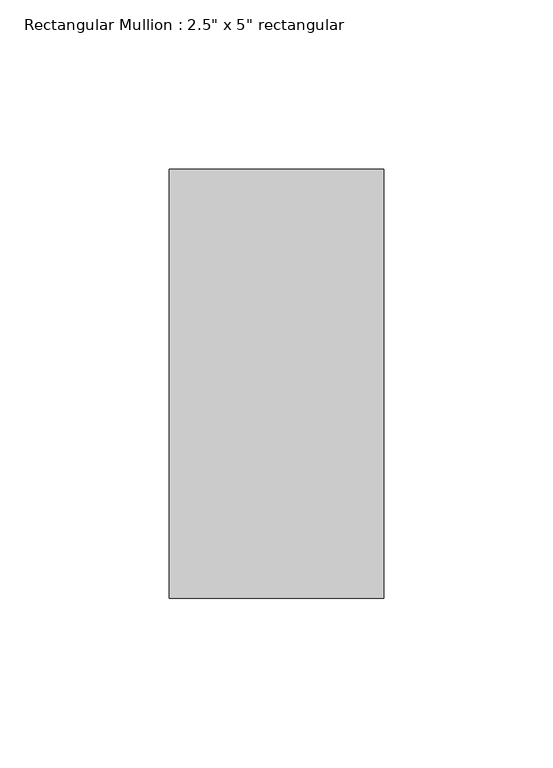
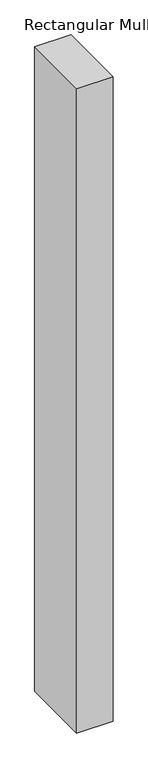
"""IFC4 building model written with IfcOpenShell, lengths in millimetres: member geometry."""

from ifc_helpers import new_model, si_unit, frame, origin, place, context, project, spatial, polyline, outline, extrude, source, transform, mapped, element, save


def member_c704a0f7(model_context):
    return source(origin(), model_context, "Body", "SweptSolid", [
        extrude(outline(polyline([(31.75, 63.5), (31.75, -63.5), (-31.75, -63.5), (-31.75, 63.5), (31.75, 63.5)])), frame((0.0, 0.0, -1190.625), z_axis=(0.0, 0.0, 1.0), x_axis=(1.0, 0.0, 0.0)), (0.0, 0.0, 1.0), 1190.625),
    ])


if __name__ == "__main__":
    model = new_model("IFC4")
    model_context = context("Model", 3, world=origin())
    ifc_project = project(units=[si_unit("LENGTHUNIT", "METRE", prefix="MILLI")], contexts=[model_context])
    site = spatial("IfcSite", under=ifc_project)
    building = spatial("IfcBuilding", under=site)
    placement = place(None, origin())
    member_shape = member_c704a0f7(model_context)
    element("IfcMember", 1, ObjectType="Rectangular Mullion : 2.5\" x 5\" rectangular", at=placement, inside=building, context=model_context, shape_type="MappedRepresentation", body=[
        mapped(member_shape, transform((0.0, 0.0, 0.0), x_axis=(1.0, 0.0, 0.0), y_axis=(0.0, 1.0, 0.0), z_axis=(0.0, 0.0, 1.0))),
    ])
    save(model, "model.ifc")

# Revit data of these elements
# Type "Rectangular Mullion : 2.5\" x 5\" rectangular"
#   built-in parameter 1007304 = 0.416667 (stored number, unit not read)
#   built-in parameter 1007301 = 0.104167 (stored number, unit not read)
#   built-in parameter 1007300 = 0.104167 (stored number, unit not read)
# Element 1 (IfcMember, "Rectangular Mullion : 2.5\" x 5\" rectangular")
#   Materials on its faces: "Aluminum"
# Materials
#   "Aluminum": class "Metal", colour RGB 247 247 247, transparency 0, Description = "Aluminum 6061", Cost = 0
